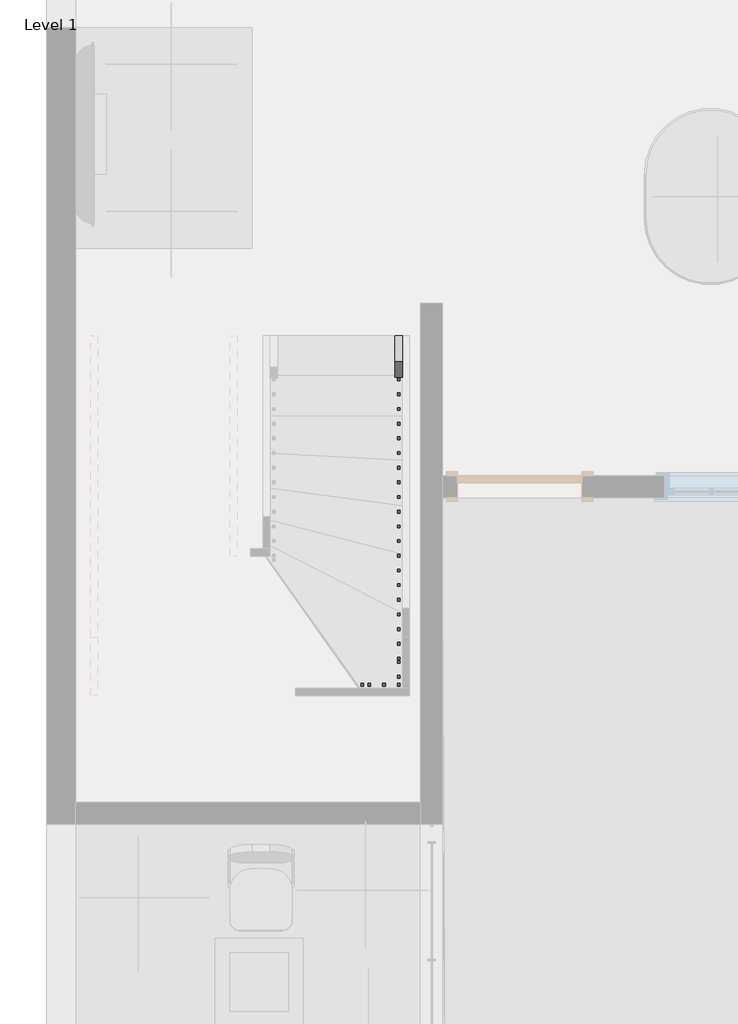
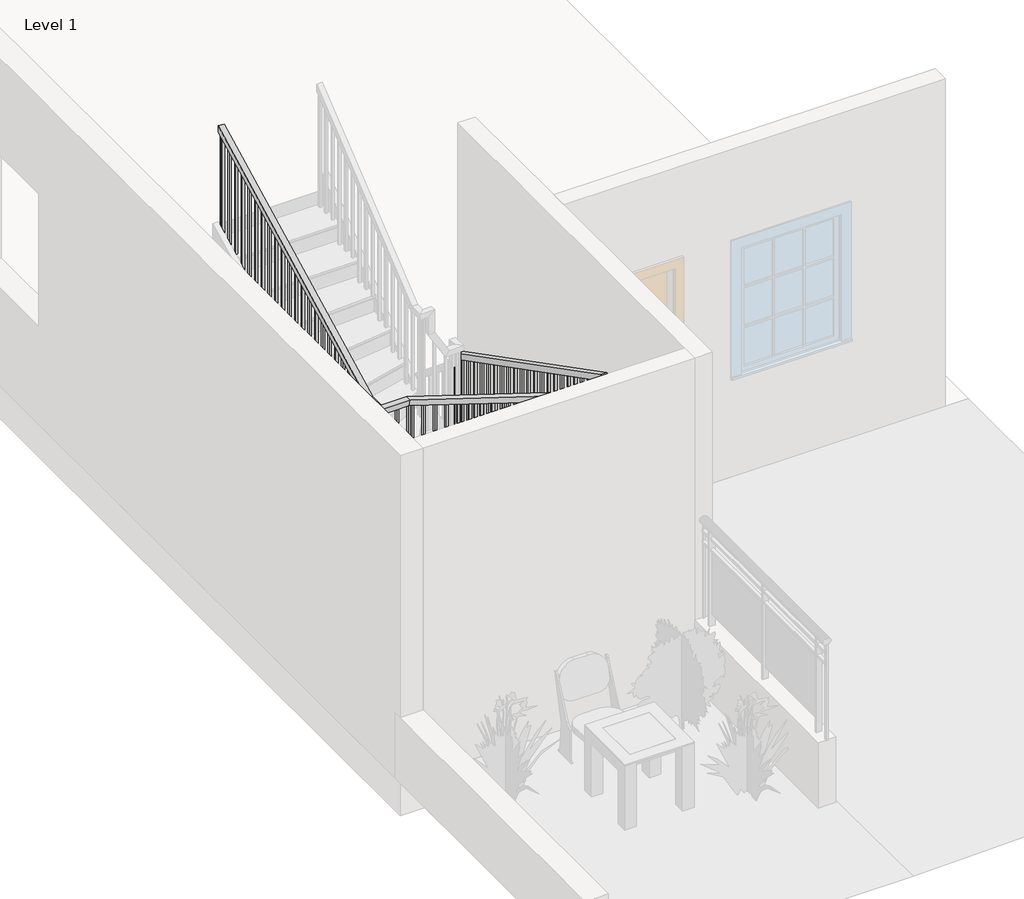
# One storey, part 2 of 3: 1 railing.
"""IFC4 building model written with IfcOpenShell, lengths in millimetres."""

from ifc_helpers import new_model, si_unit, frame, origin, place, context, project, spatial, polyline, outline, extrude, faceted_brep, element, save

model = new_model("IFC4")

# Units and contexts
model_context = context("Model", 3, world=origin())
ifc_project = project(units=[si_unit("LENGTHUNIT", "METRE", prefix="MILLI")], contexts=[model_context])

# Site, building, storey
site = spatial("IfcSite", under=ifc_project)
building = spatial("IfcBuilding", under=site)
storey = spatial("IfcBuildingStorey", under=building, Name="Level 1", Elevation=0.0)

# Railing
placement = place(None, origin())
element("IfcRailing", 1, ObjectType="Handrail - Rectangular", at=placement, inside=storey, context=model_context, shape_type="SolidModel", body=[
    faceted_brep([(-553.9479637, 880.742092, 1109.0771751), (-553.9479637, 880.742092, 1051.9280057), (-604.7479637, 880.742092, 1051.9280057), (-604.7479637, 880.742092, 1109.0771751), (-553.9479637, -1379.2397645, 2273.7644996), (-553.9479637, -1391.5598158, 2222.9644996), (-604.7479637, -1391.5598158, 2222.9644996), (-604.7479637, -1379.2397645, 2273.7644996), (-553.9479637, -1561.3895999, 2273.7644996), (-553.9479637, -1561.3895999, 2222.9644996), (-604.7479637, -1510.5895999, 2222.9644996), (-604.7479637, -1510.5895999, 2273.7644996), (-831.1019163, -1561.3895999, 2273.7644996), (-839.0524924, -1561.3895999, 2222.9644996), (-839.0524924, -1510.5895999, 2222.9644996), (-831.1019163, -1510.5895999, 2273.7644996), (-2384.9940111, -1561.3895999, 2772.3688337), (-2392.9445872, -1561.3895999, 2721.5688337), (-2392.9445872, -1510.5895999, 2721.5688337), (-2384.9940111, -1510.5895999, 2772.3688337), (-2662.1479637, -1561.3895999, 2772.3688337), (-2662.1479637, -1561.3895999, 2721.5688337), (-2611.3479637, -1510.5895999, 2721.5688337), (-2611.3479637, -1510.5895999, 2772.3688337), (-2662.1479637, -1379.2397645, 2772.3688337), (-2662.1479637, -1366.9197132, 2721.5688337), (-2611.3479637, -1366.9197132, 2721.5688337), (-2611.3479637, -1379.2397645, 2772.3688337), (-2662.1479637, 880.742092, 3937.0561582), (-2611.3479637, 880.742092, 3937.0561582), (-2611.3479637, 880.742092, 3879.9069889), (-2662.1479637, 880.742092, 3879.9069889)], [[[0, 1, 2, 3]], [[1, 0, 4, 5]], [[2, 1, 5, 6]], [[3, 2, 6, 7]], [[0, 3, 7, 4]], [[5, 4, 8, 9]], [[6, 5, 9, 10]], [[7, 6, 10, 11]], [[4, 7, 11, 8]], [[9, 8, 12, 13]], [[10, 9, 13, 14]], [[11, 10, 14, 15]], [[8, 11, 15, 12]], [[13, 12, 16, 17]], [[14, 13, 17, 18]], [[15, 14, 18, 19]], [[12, 15, 19, 16]], [[17, 16, 20, 21]], [[18, 17, 21, 22]], [[19, 18, 22, 23]], [[16, 19, 23, 20]], [[21, 20, 24, 25]], [[22, 21, 25, 26]], [[23, 22, 26, 27]], [[20, 23, 27, 24]], [[28, 29, 30, 31]], [[25, 24, 28, 31]], [[26, 25, 31, 30]], [[27, 26, 30, 29]], [[24, 27, 29, 28]]]),
    extrude(outline(polyline([(865.4852355, 3872.0443296), (865.4852355, 2878.6666667), (846.4352355, 2878.6666667), (846.4352355, 3862.2268642), (865.4852355, 3872.0443296)])), frame((-2646.2729637, 0.0, 0.0), z_axis=(1.0, 0.0, 0.0), x_axis=(0.0, 1.0, 0.0)), (0.0, 0.0, 1.0), 19.05),
    extrude(outline(polyline([(763.8852355, 3819.6845145), (763.8852355, 2878.6666667), (744.8352355, 2878.6666667), (744.8352355, 3809.8670491), (763.8852355, 3819.6845145)])), frame((-2646.2729637, 0.0, 0.0), z_axis=(1.0, 0.0, 0.0), x_axis=(0.0, 1.0, 0.0)), (0.0, 0.0, 1.0), 19.05),
    extrude(outline(polyline([(662.2852355, 3767.3246993), (662.2852355, 2878.6666667), (643.2352355, 2878.6666667), (643.2352355, 3757.507234), (662.2852355, 3767.3246993)])), frame((-2646.2729637, 0.0, 0.0), z_axis=(1.0, 0.0, 0.0), x_axis=(0.0, 1.0, 0.0)), (0.0, 0.0, 1.0), 19.05),
    extrude(outline(polyline([(560.6852355, 3714.9648842), (560.6852355, 2709.3333333), (541.6352355, 2709.3333333), (541.6352355, 3705.1474189), (560.6852355, 3714.9648842)])), frame((-2646.2729637, 0.0, 0.0), z_axis=(1.0, 0.0, 0.0), x_axis=(0.0, 1.0, 0.0)), (0.0, 0.0, 1.0), 19.05),
    extrude(outline(polyline([(459.0852355, 3662.6050691), (459.0852355, 2709.3333333), (440.0352355, 2709.3333333), (440.0352355, 3652.7876038), (459.0852355, 3662.6050691)])), frame((-2646.2729637, 0.0, 0.0), z_axis=(1.0, 0.0, 0.0), x_axis=(0.0, 1.0, 0.0)), (0.0, 0.0, 1.0), 19.05),
    extrude(outline(polyline([(357.4852355, 3610.245254), (357.4852355, 2709.3333333), (338.4352355, 2709.3333333), (338.4352355, 3600.4277887), (357.4852355, 3610.245254)])), frame((-2646.2729637, 0.0, 0.0), z_axis=(1.0, 0.0, 0.0), x_axis=(0.0, 1.0, 0.0)), (0.0, 0.0, 1.0), 19.05),
    extrude(outline(polyline([(255.8852355, 3557.8854389), (255.8852355, 2540.0), (236.8352355, 2540.0), (236.8352355, 3548.0679735), (255.8852355, 3557.8854389)])), frame((-2646.2729637, 0.0, 0.0), z_axis=(1.0, 0.0, 0.0), x_axis=(0.0, 1.0, 0.0)), (0.0, 0.0, 1.0), 19.05),
    extrude(outline(polyline([(154.2852355, 3505.5256238), (154.2852355, 2540.0), (135.2352355, 2540.0), (135.2352355, 3495.7081584), (154.2852355, 3505.5256238)])), frame((-2646.2729637, 0.0, 0.0), z_axis=(1.0, 0.0, 0.0), x_axis=(0.0, 1.0, 0.0)), (0.0, 0.0, 1.0), 19.05),
    extrude(outline(polyline([(52.6852355, 3453.1658086), (52.6852355, 2540.0), (33.6352355, 2540.0), (33.6352355, 3443.3483433), (52.6852355, 3453.1658086)])), frame((-2646.2729637, 0.0, 0.0), z_axis=(1.0, 0.0, 0.0), x_axis=(0.0, 1.0, 0.0)), (0.0, 0.0, 1.0), 19.05),
    extrude(outline(polyline([(-48.9147645, 3400.8059935), (-48.9147645, 2370.6666667), (-67.9647645, 2370.6666667), (-67.9647645, 3390.9885282), (-48.9147645, 3400.8059935)])), frame((-2646.2729637, 0.0, 0.0), z_axis=(1.0, 0.0, 0.0), x_axis=(0.0, 1.0, 0.0)), (0.0, 0.0, 1.0), 19.05),
    extrude(outline(polyline([(-150.5147645, 3348.4461784), (-150.5147645, 2370.6666667), (-169.5647645, 2370.6666667), (-169.5647645, 3338.6287131), (-150.5147645, 3348.4461784)])), frame((-2646.2729637, 0.0, 0.0), z_axis=(1.0, 0.0, 0.0), x_axis=(0.0, 1.0, 0.0)), (0.0, 0.0, 1.0), 19.05),
    extrude(outline(polyline([(-252.1147645, 3296.0863633), (-252.1147645, 2370.6666667), (-271.1647645, 2370.6666667), (-271.1647645, 3286.268898), (-252.1147645, 3296.0863633)])), frame((-2646.2729637, 0.0, 0.0), z_axis=(1.0, 0.0, 0.0), x_axis=(0.0, 1.0, 0.0)), (0.0, 0.0, 1.0), 19.05),
    extrude(outline(polyline([(-353.7147645, 3243.7265482), (-353.7147645, 2201.3333333), (-372.7647645, 2201.3333333), (-372.7647645, 3233.9090828), (-353.7147645, 3243.7265482)])), frame((-2646.2729637, 0.0, 0.0), z_axis=(1.0, 0.0, 0.0), x_axis=(0.0, 1.0, 0.0)), (0.0, 0.0, 1.0), 19.05),
    extrude(outline(polyline([(-455.3147645, 3191.3667331), (-455.3147645, 2201.3333333), (-474.3647645, 2201.3333333), (-474.3647645, 3181.5492677), (-455.3147645, 3191.3667331)])), frame((-2646.2729637, 0.0, 0.0), z_axis=(1.0, 0.0, 0.0), x_axis=(0.0, 1.0, 0.0)), (0.0, 0.0, 1.0), 19.05),
    extrude(outline(polyline([(-556.9147645, 3139.0069179), (-556.9147645, 2201.3333333), (-575.9647645, 2201.3333333), (-575.9647645, 3129.1894526), (-556.9147645, 3139.0069179)])), frame((-2646.2729637, 0.0, 0.0), z_axis=(1.0, 0.0, 0.0), x_axis=(0.0, 1.0, 0.0)), (0.0, 0.0, 1.0), 19.05),
    extrude(outline(polyline([(-658.5147645, 3086.6471028), (-658.5147645, 2032.0), (-677.5647645, 2032.0), (-677.5647645, 3076.8296375), (-658.5147645, 3086.6471028)])), frame((-2646.2729637, 0.0, 0.0), z_axis=(1.0, 0.0, 0.0), x_axis=(0.0, 1.0, 0.0)), (0.0, 0.0, 1.0), 19.05),
    extrude(outline(polyline([(-760.1147645, 3034.2872877), (-760.1147645, 2032.0), (-779.1647645, 2032.0), (-779.1647645, 3024.4698224), (-760.1147645, 3034.2872877)])), frame((-2646.2729637, 0.0, 0.0), z_axis=(1.0, 0.0, 0.0), x_axis=(0.0, 1.0, 0.0)), (0.0, 0.0, 1.0), 19.05),
    extrude(outline(polyline([(-861.7147645, 2981.9274726), (-861.7147645, 2032.0), (-880.7647645, 2032.0), (-880.7647645, 2972.1100073), (-861.7147645, 2981.9274726)])), frame((-2646.2729637, 0.0, 0.0), z_axis=(1.0, 0.0, 0.0), x_axis=(0.0, 1.0, 0.0)), (0.0, 0.0, 1.0), 19.05),
    extrude(outline(polyline([(-963.3147645, 2929.5676575), (-963.3147645, 2032.0), (-982.3647645, 2032.0), (-982.3647645, 2919.7501921), (-963.3147645, 2929.5676575)])), frame((-2646.2729637, 0.0, 0.0), z_axis=(1.0, 0.0, 0.0), x_axis=(0.0, 1.0, 0.0)), (0.0, 0.0, 1.0), 19.05),
    extrude(outline(polyline([(-1064.9147645, 2877.2078424), (-1064.9147645, 1862.6666667), (-1083.9647645, 1862.6666667), (-1083.9647645, 2867.390377), (-1064.9147645, 2877.2078424)])), frame((-2646.2729637, 0.0, 0.0), z_axis=(1.0, 0.0, 0.0), x_axis=(0.0, 1.0, 0.0)), (0.0, 0.0, 1.0), 19.05),
    extrude(outline(polyline([(-1166.5147645, 2824.8480272), (-1166.5147645, 1862.6666667), (-1185.5647645, 1862.6666667), (-1185.5647645, 2815.0305619), (-1166.5147645, 2824.8480272)])), frame((-2646.2729637, 0.0, 0.0), z_axis=(1.0, 0.0, 0.0), x_axis=(0.0, 1.0, 0.0)), (0.0, 0.0, 1.0), 19.05),
    extrude(outline(polyline([(-1268.1147645, 2772.4882121), (-1268.1147645, 1862.6666667), (-1287.1647645, 1862.6666667), (-1287.1647645, 2762.6707468), (-1268.1147645, 2772.4882121)])), frame((-2646.2729637, 0.0, 0.0), z_axis=(1.0, 0.0, 0.0), x_axis=(0.0, 1.0, 0.0)), (0.0, 0.0, 1.0), 19.05),
    extrude(outline(polyline([(-2646.2729637, -1443.9145999), (-2646.2729637, -1424.8645999), (-2627.2229637, -1424.8645999), (-2627.2229637, -1443.9145999), (-2646.2729637, -1443.9145999)])), frame((0.0, 0.0, 1862.6666667), z_axis=(0.0, 0.0, 1.0), x_axis=(1.0, 0.0, 0.0)), (0.0, 0.0, 1.0), 858.902167),
    extrude(outline(polyline([(-2578.6690111, -1545.5145999), (-2597.7190111, -1545.5145999), (-2597.7190111, -1526.4645999), (-2578.6690111, -1526.4645999), (-2578.6690111, -1545.5145999)])), frame((0.0, 0.0, 1862.6666667), z_axis=(0.0, 0.0, 1.0), x_axis=(1.0, 0.0, 0.0)), (0.0, 0.0, 1.0), 858.902167),
    extrude(outline(polyline([(-2477.0690111, -1545.5145999), (-2496.1190111, -1545.5145999), (-2496.1190111, -1526.4645999), (-2477.0690111, -1526.4645999), (-2477.0690111, -1545.5145999)])), frame((0.0, 0.0, 1862.6666667), z_axis=(0.0, 0.0, 1.0), x_axis=(1.0, 0.0, 0.0)), (0.0, 0.0, 1.0), 858.902167),
    extrude(outline(polyline([(2712.4824155, -2364.6269163), (1693.3333333, -2364.6269163), (1693.3333333, -2345.5769163), (2706.3697564, -2345.5769163), (2712.4824155, -2364.6269163)])), frame((0.0, -1545.5145999, 0.0), z_axis=(0.0, 1.0, 0.0), x_axis=(0.0, 0.0, 1.0)), (0.0, 0.0, 1.0), 19.05),
    extrude(outline(polyline([(2679.8815673, -2263.0269163), (1693.3333333, -2263.0269163), (1693.3333333, -2243.9769163), (2673.7689082, -2243.9769163), (2679.8815673, -2263.0269163)])), frame((0.0, -1545.5145999, 0.0), z_axis=(0.0, 1.0, 0.0), x_axis=(0.0, 0.0, 1.0)), (0.0, 0.0, 1.0), 19.05),
    extrude(outline(polyline([(2647.280719, -2161.4269163), (1693.3333333, -2161.4269163), (1693.3333333, -2142.3769163), (2641.16806, -2142.3769163), (2647.280719, -2161.4269163)])), frame((0.0, -1545.5145999, 0.0), z_axis=(0.0, 1.0, 0.0), x_axis=(0.0, 0.0, 1.0)), (0.0, 0.0, 1.0), 19.05),
    extrude(outline(polyline([(2614.6798708, -2059.8269163), (1693.3333333, -2059.8269163), (1693.3333333, -2040.7769163), (2608.5672118, -2040.7769163), (2614.6798708, -2059.8269163)])), frame((0.0, -1545.5145999, 0.0), z_axis=(0.0, 1.0, 0.0), x_axis=(0.0, 0.0, 1.0)), (0.0, 0.0, 1.0), 19.05),
    extrude(outline(polyline([(2582.0790226, -1958.2269163), (1693.3333333, -1958.2269163), (1693.3333333, -1939.1769163), (2575.9663635, -1939.1769163), (2582.0790226, -1958.2269163)])), frame((0.0, -1545.5145999, 0.0), z_axis=(0.0, 1.0, 0.0), x_axis=(0.0, 0.0, 1.0)), (0.0, 0.0, 1.0), 19.05),
    extrude(outline(polyline([(2549.4781744, -1856.6269163), (1693.3333333, -1856.6269163), (1693.3333333, -1837.5769163), (2543.3655153, -1837.5769163), (2549.4781744, -1856.6269163)])), frame((0.0, -1545.5145999, 0.0), z_axis=(0.0, 1.0, 0.0), x_axis=(0.0, 0.0, 1.0)), (0.0, 0.0, 1.0), 19.05),
    extrude(outline(polyline([(2516.8773261, -1755.0269163), (1524.0, -1755.0269163), (1524.0, -1735.9769163), (2510.7646671, -1735.9769163), (2516.8773261, -1755.0269163)])), frame((0.0, -1545.5145999, 0.0), z_axis=(0.0, 1.0, 0.0), x_axis=(0.0, 0.0, 1.0)), (0.0, 0.0, 1.0), 19.05),
    extrude(outline(polyline([(2484.2764779, -1653.4269163), (1524.0, -1653.4269163), (1524.0, -1634.3769163), (2478.1638189, -1634.3769163), (2484.2764779, -1653.4269163)])), frame((0.0, -1545.5145999, 0.0), z_axis=(0.0, 1.0, 0.0), x_axis=(0.0, 0.0, 1.0)), (0.0, 0.0, 1.0), 19.05),
    extrude(outline(polyline([(2451.6756297, -1551.8269163), (1524.0, -1551.8269163), (1524.0, -1532.7769163), (2445.5629706, -1532.7769163), (2451.6756297, -1551.8269163)])), frame((0.0, -1545.5145999, 0.0), z_axis=(0.0, 1.0, 0.0), x_axis=(0.0, 0.0, 1.0)), (0.0, 0.0, 1.0), 19.05),
    extrude(outline(polyline([(2419.0747814, -1450.2269163), (1524.0, -1450.2269163), (1524.0, -1431.1769163), (2412.9621224, -1431.1769163), (2419.0747814, -1450.2269163)])), frame((0.0, -1545.5145999, 0.0), z_axis=(0.0, 1.0, 0.0), x_axis=(0.0, 0.0, 1.0)), (0.0, 0.0, 1.0), 19.05),
    extrude(outline(polyline([(2386.4739332, -1348.6269163), (1354.6666667, -1348.6269163), (1354.6666667, -1329.5769163), (2380.3612742, -1329.5769163), (2386.4739332, -1348.6269163)])), frame((0.0, -1545.5145999, 0.0), z_axis=(0.0, 1.0, 0.0), x_axis=(0.0, 0.0, 1.0)), (0.0, 0.0, 1.0), 19.05),
    extrude(outline(polyline([(2353.873085, -1247.0269163), (1354.6666667, -1247.0269163), (1354.6666667, -1227.9769163), (2347.7604259, -1227.9769163), (2353.873085, -1247.0269163)])), frame((0.0, -1545.5145999, 0.0), z_axis=(0.0, 1.0, 0.0), x_axis=(0.0, 0.0, 1.0)), (0.0, 0.0, 1.0), 19.05),
    extrude(outline(polyline([(2321.2722368, -1145.4269163), (1354.6666667, -1145.4269163), (1354.6666667, -1126.3769163), (2315.1595777, -1126.3769163), (2321.2722368, -1145.4269163)])), frame((0.0, -1545.5145999, 0.0), z_axis=(0.0, 1.0, 0.0), x_axis=(0.0, 0.0, 1.0)), (0.0, 0.0, 1.0), 19.05),
    extrude(outline(polyline([(2288.6713885, -1043.8269163), (1354.6666667, -1043.8269163), (1354.6666667, -1024.7769163), (2282.5587295, -1024.7769163), (2288.6713885, -1043.8269163)])), frame((0.0, -1545.5145999, 0.0), z_axis=(0.0, 1.0, 0.0), x_axis=(0.0, 0.0, 1.0)), (0.0, 0.0, 1.0), 19.05),
    extrude(outline(polyline([(2256.0705403, -942.2269163), (1354.6666667, -942.2269163), (1354.6666667, -923.1769163), (2249.9578813, -923.1769163), (2256.0705403, -942.2269163)])), frame((0.0, -1545.5145999, 0.0), z_axis=(0.0, 1.0, 0.0), x_axis=(0.0, 0.0, 1.0)), (0.0, 0.0, 1.0), 19.05),
    extrude(outline(polyline([(-773.0229637, -1545.5145999), (-792.0729637, -1545.5145999), (-792.0729637, -1526.4645999), (-773.0229637, -1526.4645999), (-773.0229637, -1545.5145999)])), frame((0.0, 0.0, 1185.3333333), z_axis=(0.0, 0.0, 1.0), x_axis=(1.0, 0.0, 0.0)), (0.0, 0.0, 1.0), 1037.6311663),
    extrude(outline(polyline([(-671.4229637, -1545.5145999), (-690.4729637, -1545.5145999), (-690.4729637, -1526.4645999), (-671.4229637, -1526.4645999), (-671.4229637, -1545.5145999)])), frame((0.0, 0.0, 1185.3333333), z_axis=(0.0, 0.0, 1.0), x_axis=(1.0, 0.0, 0.0)), (0.0, 0.0, 1.0), 1037.6311663),
    extrude(outline(polyline([(-569.8229637, -1471.3147645), (-569.8229637, -1490.3647645), (-588.8729637, -1490.3647645), (-588.8729637, -1471.3147645), (-569.8229637, -1471.3147645)])), frame((0.0, 0.0, 1185.3333333), z_axis=(0.0, 0.0, 1.0), x_axis=(1.0, 0.0, 0.0)), (0.0, 0.0, 1.0), 1037.6311663),
    extrude(outline(polyline([(-1344.932908, 2198.9352056), (-1344.932908, 1185.3333333), (-1363.982908, 1185.3333333), (-1363.982908, 2208.752671), (-1344.932908, 2198.9352056)])), frame((-588.8729637, 0.0, 0.0), z_axis=(1.0, 0.0, 0.0), x_axis=(0.0, 1.0, 0.0)), (0.0, 0.0, 1.0), 19.05),
    extrude(outline(polyline([(-1243.332908, 2146.5753905), (-1243.332908, 1185.3333333), (-1262.382908, 1185.3333333), (-1262.382908, 2156.3928558), (-1243.332908, 2146.5753905)])), frame((-588.8729637, 0.0, 0.0), z_axis=(1.0, 0.0, 0.0), x_axis=(0.0, 1.0, 0.0)), (0.0, 0.0, 1.0), 19.05),
    extrude(outline(polyline([(-1141.732908, 2094.2155754), (-1141.732908, 1185.3333333), (-1160.782908, 1185.3333333), (-1160.782908, 2104.0330407), (-1141.732908, 2094.2155754)])), frame((-588.8729637, 0.0, 0.0), z_axis=(1.0, 0.0, 0.0), x_axis=(0.0, 1.0, 0.0)), (0.0, 0.0, 1.0), 19.05),
    extrude(outline(polyline([(-1040.132908, 2041.8557603), (-1040.132908, 1185.3333333), (-1059.182908, 1185.3333333), (-1059.182908, 2051.6732256), (-1040.132908, 2041.8557603)])), frame((-588.8729637, 0.0, 0.0), z_axis=(1.0, 0.0, 0.0), x_axis=(0.0, 1.0, 0.0)), (0.0, 0.0, 1.0), 19.05),
    extrude(outline(polyline([(-938.532908, 1989.4959452), (-938.532908, 1016.0), (-957.582908, 1016.0), (-957.582908, 1999.3134105), (-938.532908, 1989.4959452)])), frame((-588.8729637, 0.0, 0.0), z_axis=(1.0, 0.0, 0.0), x_axis=(0.0, 1.0, 0.0)), (0.0, 0.0, 1.0), 19.05),
    extrude(outline(polyline([(-836.932908, 1937.13613), (-836.932908, 1016.0), (-855.982908, 1016.0), (-855.982908, 1946.9535954), (-836.932908, 1937.13613)])), frame((-588.8729637, 0.0, 0.0), z_axis=(1.0, 0.0, 0.0), x_axis=(0.0, 1.0, 0.0)), (0.0, 0.0, 1.0), 19.05),
    extrude(outline(polyline([(-735.332908, 1884.7763149), (-735.332908, 1016.0), (-754.382908, 1016.0), (-754.382908, 1894.5937803), (-735.332908, 1884.7763149)])), frame((-588.8729637, 0.0, 0.0), z_axis=(1.0, 0.0, 0.0), x_axis=(0.0, 1.0, 0.0)), (0.0, 0.0, 1.0), 19.05),
    extrude(outline(polyline([(-633.732908, 1832.4164998), (-633.732908, 1016.0), (-652.782908, 1016.0), (-652.782908, 1842.2339651), (-633.732908, 1832.4164998)])), frame((-588.8729637, 0.0, 0.0), z_axis=(1.0, 0.0, 0.0), x_axis=(0.0, 1.0, 0.0)), (0.0, 0.0, 1.0), 19.05),
    extrude(outline(polyline([(-532.132908, 1780.0566847), (-532.132908, 846.6666667), (-551.182908, 846.6666667), (-551.182908, 1789.87415), (-532.132908, 1780.0566847)])), frame((-588.8729637, 0.0, 0.0), z_axis=(1.0, 0.0, 0.0), x_axis=(0.0, 1.0, 0.0)), (0.0, 0.0, 1.0), 19.05),
    extrude(outline(polyline([(-430.532908, 1727.6968696), (-430.532908, 846.6666667), (-449.582908, 846.6666667), (-449.582908, 1737.5143349), (-430.532908, 1727.6968696)])), frame((-588.8729637, 0.0, 0.0), z_axis=(1.0, 0.0, 0.0), x_axis=(0.0, 1.0, 0.0)), (0.0, 0.0, 1.0), 19.05),
    extrude(outline(polyline([(-328.932908, 1675.3370545), (-328.932908, 846.6666667), (-347.982908, 846.6666667), (-347.982908, 1685.1545198), (-328.932908, 1675.3370545)])), frame((-588.8729637, 0.0, 0.0), z_axis=(1.0, 0.0, 0.0), x_axis=(0.0, 1.0, 0.0)), (0.0, 0.0, 1.0), 19.05),
    extrude(outline(polyline([(-227.332908, 1622.9772393), (-227.332908, 677.3333333), (-246.382908, 677.3333333), (-246.382908, 1632.7947047), (-227.332908, 1622.9772393)])), frame((-588.8729637, 0.0, 0.0), z_axis=(1.0, 0.0, 0.0), x_axis=(0.0, 1.0, 0.0)), (0.0, 0.0, 1.0), 19.05),
    extrude(outline(polyline([(-125.732908, 1570.6174242), (-125.732908, 677.3333333), (-144.782908, 677.3333333), (-144.782908, 1580.4348896), (-125.732908, 1570.6174242)])), frame((-588.8729637, 0.0, 0.0), z_axis=(1.0, 0.0, 0.0), x_axis=(0.0, 1.0, 0.0)), (0.0, 0.0, 1.0), 19.05),
    extrude(outline(polyline([(-24.132908, 1518.2576091), (-24.132908, 677.3333333), (-43.182908, 677.3333333), (-43.182908, 1528.0750744), (-24.132908, 1518.2576091)])), frame((-588.8729637, 0.0, 0.0), z_axis=(1.0, 0.0, 0.0), x_axis=(0.0, 1.0, 0.0)), (0.0, 0.0, 1.0), 19.05),
    extrude(outline(polyline([(77.467092, 1465.897794), (77.467092, 508.0), (58.417092, 508.0), (58.417092, 1475.7152593), (77.467092, 1465.897794)])), frame((-588.8729637, 0.0, 0.0), z_axis=(1.0, 0.0, 0.0), x_axis=(0.0, 1.0, 0.0)), (0.0, 0.0, 1.0), 19.05),
    extrude(outline(polyline([(179.067092, 1413.5379789), (179.067092, 508.0), (160.017092, 508.0), (160.017092, 1423.3554442), (179.067092, 1413.5379789)])), frame((-588.8729637, 0.0, 0.0), z_axis=(1.0, 0.0, 0.0), x_axis=(0.0, 1.0, 0.0)), (0.0, 0.0, 1.0), 19.05),
    extrude(outline(polyline([(280.667092, 1361.1781638), (280.667092, 508.0), (261.617092, 508.0), (261.617092, 1370.9956291), (280.667092, 1361.1781638)])), frame((-588.8729637, 0.0, 0.0), z_axis=(1.0, 0.0, 0.0), x_axis=(0.0, 1.0, 0.0)), (0.0, 0.0, 1.0), 19.05),
    extrude(outline(polyline([(382.267092, 1308.8183486), (382.267092, 338.6666667), (363.217092, 338.6666667), (363.217092, 1318.635814), (382.267092, 1308.8183486)])), frame((-588.8729637, 0.0, 0.0), z_axis=(1.0, 0.0, 0.0), x_axis=(0.0, 1.0, 0.0)), (0.0, 0.0, 1.0), 19.05),
    extrude(outline(polyline([(483.867092, 1256.4585335), (483.867092, 338.6666667), (464.817092, 338.6666667), (464.817092, 1266.2759989), (483.867092, 1256.4585335)])), frame((-588.8729637, 0.0, 0.0), z_axis=(1.0, 0.0, 0.0), x_axis=(0.0, 1.0, 0.0)), (0.0, 0.0, 1.0), 19.05),
    extrude(outline(polyline([(585.467092, 1204.0987184), (585.467092, 338.6666667), (566.417092, 338.6666667), (566.417092, 1213.9161837), (585.467092, 1204.0987184)])), frame((-588.8729637, 0.0, 0.0), z_axis=(1.0, 0.0, 0.0), x_axis=(0.0, 1.0, 0.0)), (0.0, 0.0, 1.0), 19.05),
    extrude(outline(polyline([(687.067092, 1151.7389033), (687.067092, 169.3333333), (668.017092, 169.3333333), (668.017092, 1161.5563686), (687.067092, 1151.7389033)])), frame((-588.8729637, 0.0, 0.0), z_axis=(1.0, 0.0, 0.0), x_axis=(0.0, 1.0, 0.0)), (0.0, 0.0, 1.0), 19.05),
    extrude(outline(polyline([(788.667092, 1099.3790882), (788.667092, 169.3333333), (769.617092, 169.3333333), (769.617092, 1109.1965535), (788.667092, 1099.3790882)])), frame((-588.8729637, 0.0, 0.0), z_axis=(1.0, 0.0, 0.0), x_axis=(0.0, 1.0, 0.0)), (0.0, 0.0, 1.0), 19.05),
    extrude(outline(polyline([(-2646.2729637, -1388.7647645), (-2646.2729637, -1369.7147645), (-2627.2229637, -1369.7147645), (-2627.2229637, -1388.7647645), (-2646.2729637, -1388.7647645)])), frame((0.0, 0.0, 1862.6666667), z_axis=(0.0, 0.0, 1.0), x_axis=(1.0, 0.0, 0.0)), (0.0, 0.0, 1.0), 858.902167),
    extrude(outline(polyline([(-2627.2229637, -1545.5145999), (-2646.2729637, -1545.5145999), (-2646.2729637, -1526.4645999), (-2627.2229637, -1526.4645999), (-2627.2229637, -1545.5145999)])), frame((0.0, 0.0, 1862.6666667), z_axis=(0.0, 0.0, 1.0), x_axis=(1.0, 0.0, 0.0)), (0.0, 0.0, 1.0), 858.902167),
    extrude(outline(polyline([(2722.0740262, -2394.5190111), (1862.6666667, -2394.5190111), (1862.6666667, -2375.4690111), (2715.9613671, -2375.4690111), (2722.0740262, -2394.5190111)])), frame((0.0, -1545.5145999, 0.0), z_axis=(0.0, 1.0, 0.0), x_axis=(0.0, 0.0, 1.0)), (0.0, 0.0, 1.0), 19.05),
    extrude(outline(polyline([(-821.5769163, -1545.5145999), (-840.6269163, -1545.5145999), (-840.6269163, -1526.4645999), (-821.5769163, -1526.4645999), (-821.5769163, -1545.5145999)])), frame((0.0, 0.0, 1185.3333333), z_axis=(0.0, 0.0, 1.0), x_axis=(1.0, 0.0, 0.0)), (0.0, 0.0, 1.0), 1037.6311663),
    extrude(outline(polyline([(-569.8229637, -1526.4645999), (-569.8229637, -1545.5145999), (-588.8729637, -1545.5145999), (-588.8729637, -1526.4645999), (-569.8229637, -1526.4645999)])), frame((0.0, 0.0, 1185.3333333), z_axis=(0.0, 0.0, 1.0), x_axis=(1.0, 0.0, 0.0)), (0.0, 0.0, 1.0), 1037.6311663),
    extrude(outline(polyline([(-1369.7147645, 2211.7065976), (-1369.7147645, 1185.3333333), (-1388.7647645, 1185.3333333), (-1388.7647645, 2221.5240629), (-1369.7147645, 2211.7065976)])), frame((-588.8729637, 0.0, 0.0), z_axis=(1.0, 0.0, 0.0), x_axis=(0.0, 1.0, 0.0)), (0.0, 0.0, 1.0), 19.05),
    extrude(outline(polyline([(880.742092, 3879.9069889), (880.742092, 2878.6666667), (861.692092, 2878.6666667), (861.692092, 3870.0895235), (880.742092, 3879.9069889)])), frame((-2646.2729637, 0.0, 0.0), z_axis=(1.0, 0.0, 0.0), x_axis=(0.0, 1.0, 0.0)), (0.0, 0.0, 1.0), 19.05),
    extrude(outline(polyline([(880.742092, 1051.9280057), (880.742092, 169.3333333), (861.692092, 169.3333333), (861.692092, 1061.7454711), (880.742092, 1051.9280057)])), frame((-588.8729637, 0.0, 0.0), z_axis=(1.0, 0.0, 0.0), x_axis=(0.0, 1.0, 0.0)), (0.0, 0.0, 1.0), 19.05),
])

save(model, "model.ifc")

# Revit data of these elements
# Type "Handrail - Rectangular"
#   Assembly Code = "C2010400"
#   built-in parameter 1008612 = 0.0416667 (stored number, unit not read)
#   built-in parameter 1008611 = 0.0416667 (stored number, unit not read)
#   built-in parameter 1008609 = 0.333333 (stored number, unit not read)
#   built-in parameter 1008604 = 0.166667 (stored number, unit not read)
#   built-in parameter 1008603 = 0.166667 (stored number, unit not read)
#   Railing Height = 3' - 0"
#   built-in parameter 1008630 = 2
#   built-in parameter 1008610 = 2
#   built-in parameter 1008618 = Baluster - Square : 3/4"
# Element 1 (IfcRailing, "Handrail - Rectangular")
#   Phase Created = New Construction
